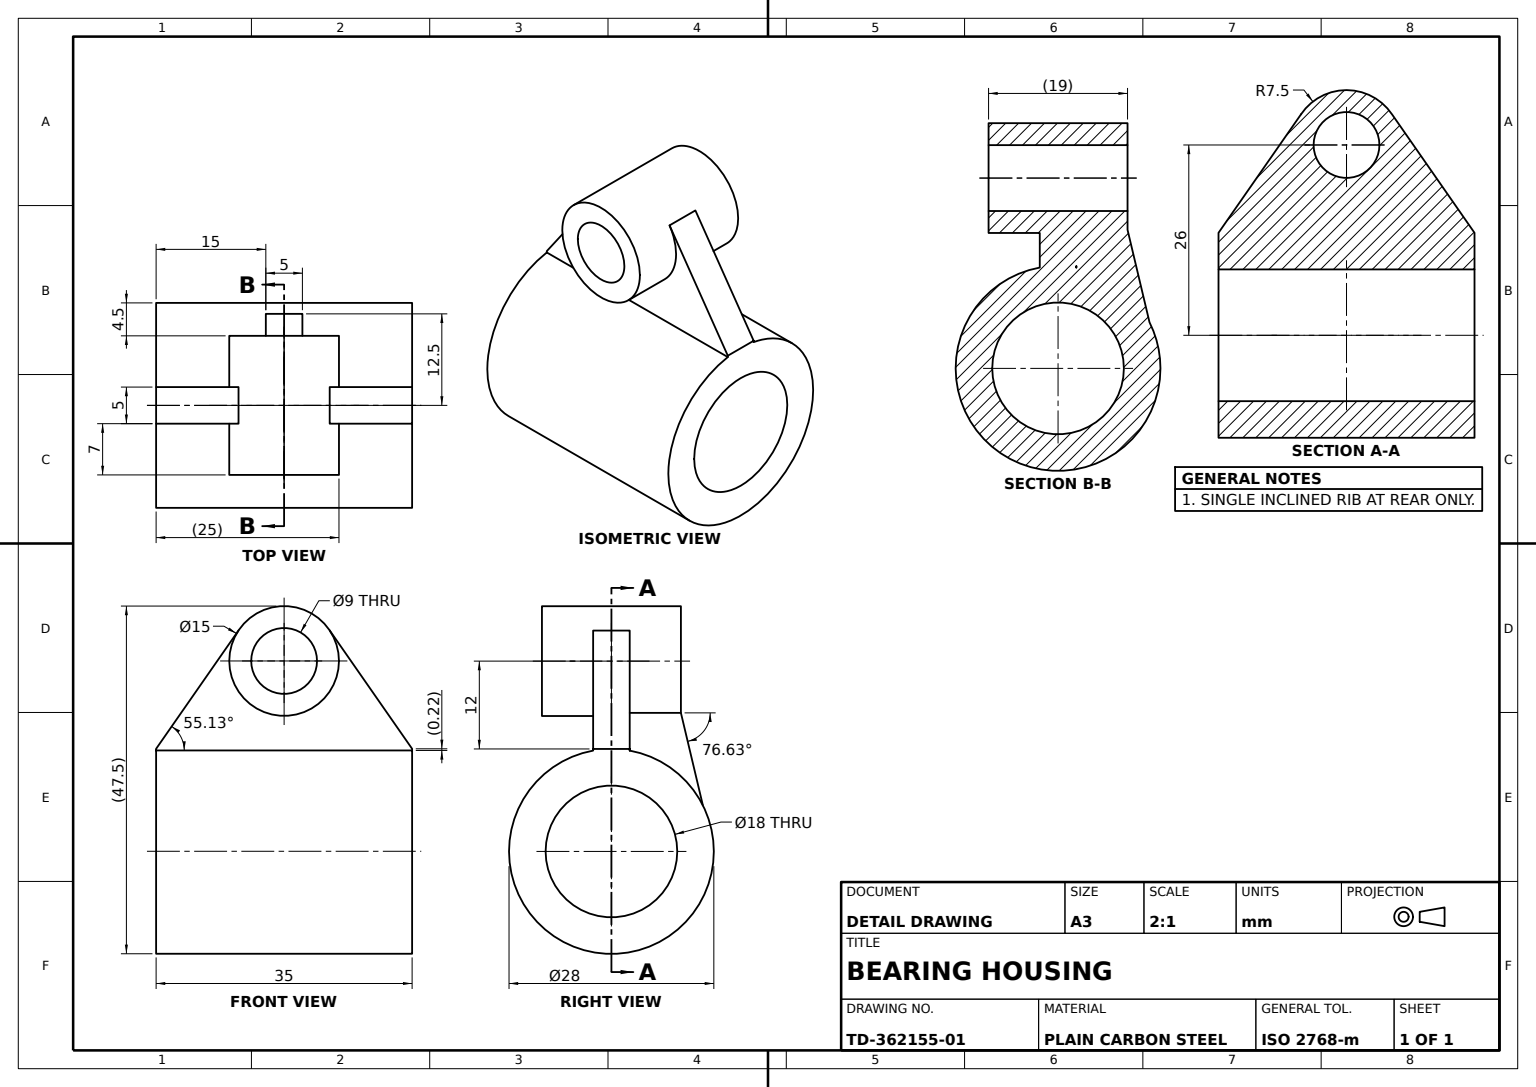
SolidWorks part; units mm, degrees
material "Plain Carbon Steel"
ref_plane "Front Plane" through (0, 0, 0) normal (0, 0, 1) x (1, 0, 0)
ref_plane "Top Plane" through (0, 0, 0) normal (0, 1, 0) x (1, 0, 0)
ref_plane "Right Plane" through (0, 0, 0) normal (1, 0, 0) x (0, 0, -1)
sketch "Main Cylinder Sketch" plane through (0, 0, 0) normal (0, 0, 1) x (1, 0, 0)
  circle A0 centre (0, 0) radius 14
  dimension "D1" = 28
extrude "Main Cylinder Ø28" add sketch "Main Cylinder Sketch" against normal blind 35
sketch "Main Bore Sketch" plane through (0, 0, 0) normal (0, 0, 1) x (1, 0, 0)
  circle A0 centre (0, 0) radius 9
  dimension "D1" = 18
extrude "Main Bore Ø18" cut sketch "Main Bore Sketch" against normal blind 35
ref_plane "Plane1" through (0, 0, 0) normal (1, 0, 0) x (0, 0, -1)
sketch "Base Web Sketch" plane through (0, 0, 0) normal (1, 0, 0) x (0, 0, -1)
  line L3 (25, 26) -> (35, 14)
  line L4 (35, 14) -> (0, 14)
  line L5 (10, 26) -> (0, 14)
  circle A0 centre (17.5, 26) radius 7.5
  dimension "D5" = 15
  dimension "D1" = 12
  dimension "D2" = 7.5
  dimension "D3" = 7.5
  dimension "D4" = 25
  dimension "D6" = 12
  dimension "D7" = 17.5
extrude "Base Web" add sketch "Base Web Sketch" against normal blind 2.5 separate body contours A0 | A0 L5 L4 L3
sketch "Second Web Sketch" plane through (0, 0, 0) normal (1, 0, 0) x (0, 0, -1)
  line L0 (0, 14) -> (35, 14)
  line L1 (35, 14) -> (25, 26)
  line L2 (0, 14) -> (10, 26)
  circle A0 centre (17.5, 26) radius 7.5
  arc M1 (25, 26) -> (10, 26) centre (17.5, 26) ccw
  line M2 (10, 26) -> (0, 14)
  line M3 (0, 14) -> (35, 14)
  line M4 (35, 14) -> (25, 26)
  dimension "D1" = 15
extrude "Second Web" add sketch "Second Web Sketch" along normal blind 2.5 contours A0 M1 | A0 M2 M3 M4
sketch "Support Rib Sketch" plane through (2.5, 0, 0) normal (1, 0, 0) x (0, 0, -1)
  line L0 (0, 14) -> (11.4271, 30.4011)
  line L1 (0, 14) -> (10, 26)
  line L2 (35, 14) -> (23.5729, 30.4011)
  line L3 (35, 14) -> (25, 26)
  line L4 (10, 26) -> (0, 14)
  line L5 (0, 14) -> (35, 14)
  line L6 (35, 14) -> (25, 26)
  line L7 (10, 26) -> (0, 14)
  arc A0 (25, 26) -> (10, 26) centre (17.5, 26) ccw construction
  arc A1 (25, 26) -> (23.5729, 30.4011) centre (17.5, 26) ccw
  arc A2 (25, 26) -> (10, 26) centre (17.5, 26) ccw
  arc A3 (11.4271, 30.4011) -> (10, 26) centre (17.5, 26) ccw
  arc A4 (11.4271, 30.4011) -> (10, 26) centre (17.5, 26) ccw
  arc M6 (25, 26) -> (10, 26) centre (17.5, 26) ccw
  line M7 (10, 26) -> (0, 14)
  line M9 (35, 14) -> (25, 26)
  dimension "D3" = 16.4011
  dimension "D1" = 0
  dimension "D2" = 11.4271
extrude "Support Rib" add sketch "Support Rib Sketch" against normal blind 5 contours L0 M7 M6 | L2 M9 M6
sketch "Upper Boss A Sketch" plane through (2.5, 0, 0) normal (1, 0, 0) x (0, 0, -1)
  circle A0 centre (17.5, 26) radius 7.5
  dimension "D1" = 15
extrude "Upper Boss A Ø15" add sketch "Upper Boss A Sketch" along normal blind 7
sketch "Upper Boss B Sketch" plane through (-2.5, 0, 0) normal (-1, 0, 0) x (0, 0, 1)
  circle A0 centre (-17.5, 26) radius 7.5
  dimension "D1" = 15
extrude "Upper Boss B Ø15" add sketch "Upper Boss B Sketch" along normal blind 7
sketch "Boss Arm Sketch" plane through (9.5, 0, 0) normal (1, 0, 0) x (0, 0, -1)
  line L0 (15, 18.5) -> (15, 18.9289)
  line L1 (15, 18.5) -> (15, 0)
  line L2 (15, 0) -> (20, 0)
  line L3 (20, 0) -> (20, 18.9289)
  circle A0 centre (17.5, 26) radius 7.5 construction
  arc A1 (15, 18.9289) -> (20, 18.9289) centre (17.5, 26) ccw
  dimension "D1" = 15
  dimension "D2" = 5
  dimension "D3" = 7.5
extrude "Boss Arm" add sketch "Boss Arm Sketch" against normal blind 7 separate body
sketch "Saddle Fill Sketch" plane through (0, 0, 0) normal (0, 0, 1) x (1, 0, 0)
  line L0 (9.5, 18.9289) -> (12.5022, 6.3004)
  line L1 (9.5, 18.9289) -> (2.5, 18.9289)
  line L2 (2.5, 18.9289) -> (2.5, 13.775)
  line L3 (2.5, 18.9289) -> (2.5, 0) construction
  circle A0 centre (0, 0) radius 14 construction
  arc A1 (12.5022, 6.3004) -> (2.5, 13.775) centre (0, 0) ccw
  circle A2 centre (0, 0) radius 9 construction
  dimension "D1" = 12.5022
extrude "Saddle Fill" add sketch "Saddle Fill Sketch" against normal blind 35 separate body
sketch "Trim Cut 1 Sketch" plane through (0, 0, 0) normal (0, 0, 1) x (1, 0, 0)
  line L0 (2.5, 18.9289) -> (9.5, 18.9289)
  line L1 (9.5, 18.9289) -> (12.5022, 6.3004)
  line L2 (2.5, 18.9289) -> (2.5, 13.775)
  arc A0 (12.5022, 6.3004) -> (2.5, 13.775) centre (0, 0) ccw
extrude "Trim Cut 1" cut sketch "Trim Cut 1 Sketch" against normal blind 15
sketch "Trim Cut 2 Sketch" plane through (0, 0, -35) normal (0, 0, -1) x (-1, 0, 0)
  line L0 (-9.5, 18.9289) -> (-2.5, 18.9289)
  line L1 (-2.5, 18.9289) -> (-2.5, 13.775)
  line L2 (-9.5, 18.9289) -> (-12.5022, 6.3004)
extrude "Trim Cut 2" cut sketch "Trim Cut 2 Sketch" against normal blind 15 and the other way through all
sketch "Trim Cut 3 Sketch" plane through (0, 0, -15) normal (0, 0, 1) x (1, 0, 0)
  line L0 (2.5, 0) -> (9, 0)
  line L1 (2.5, 0) -> (2.5, 8.6458)
  line L2 (2.5, 18.9289) -> (2.5, 0) construction
  circle A0 centre (0, 0) radius 9 construction
  arc A1 (9, 0) -> (2.5, 8.6458) centre (0, 0) ccw
extrude "Trim Cut 3" cut sketch "Trim Cut 3 Sketch" against normal blind 15
sketch "Upper Bore Sketch" plane through (9.5, 0, 0) normal (1, 0, 0) x (0, 0, -1)
  circle A0 centre (17.5, 26) radius 4.5
  dimension "D1" = 9
extrude "Upper Bore Ø9" cut sketch "Upper Bore Sketch" against normal blind 50
sketch "Cylinder Skin Sketch" plane through (0, 0, 0) normal (0, 0, 1) x (1, 0, 0)
  line L0 (-2.5, 14) -> (-2.5, 13.775)
  line L2 (2.4955, 13.7758) -> (2.5, 14)
  line L3 (2.5, 14) -> (-2.5, 14)
  arc A0 (2.4955, 13.7758) -> (-2.5, 13.775) centre (0, 0) ccw
  circle M3 centre (0, 0) radius 14
  dimension "D1" = 28
  dimension "D2" = 0.2242
extrude "Cylinder Skin Ø28" add sketch "Cylinder Skin Sketch" against normal blind 35 contours L2 L3 M3 | L3 L0 M3
